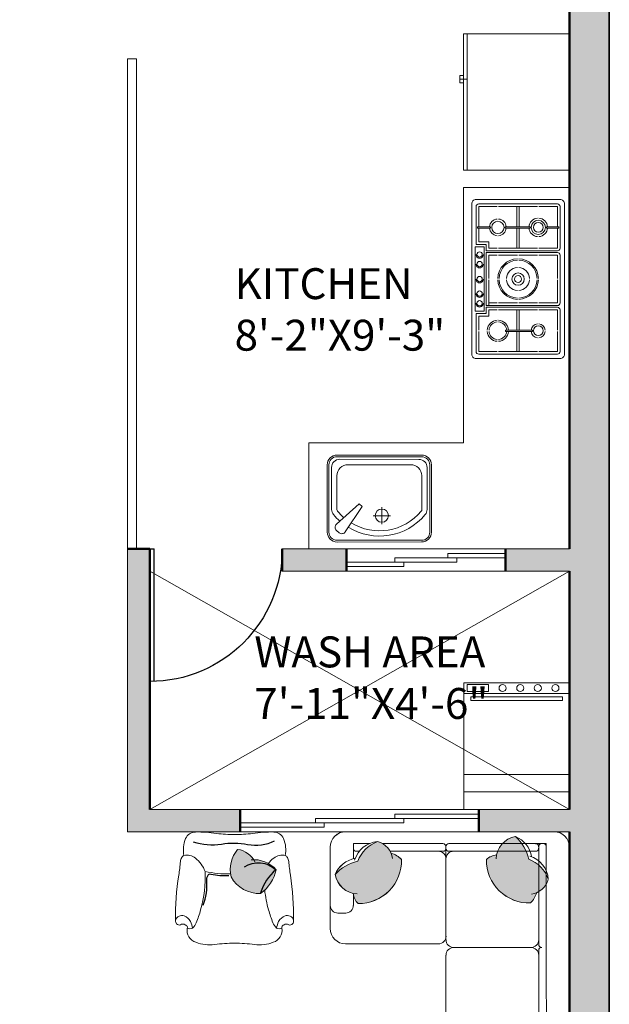
# Model space of a CAD drawing. Units: inches. Extents: x 1734 to 4011, y 1071 to 1891.
# Tile 17 of 27: x 3343 to 3476, y 1415 to 1638. Entities that reach past the tile are written whole.
import ezdxf

# ---------------------------------------------------------------- set-up
doc = ezdxf.new("R2010")
doc.units = ezdxf.units.IN
for name, color, linetype, lineweight in [('A-AREA-IDEN', 3, 'Continuous', 18), ('A-DOOR', 3, 'Continuous', 25), ('A-EQPM', 8, 'Continuous', 18), ('A-FLOR-FIXT', 9, 'Continuous', 18), ('A-FURN', 8, 'Continuous', 18), ('A-FURN-PATT', 252, 'Continuous', 13), ('A-GLAZ', 4, 'Continuous', 18), ('A-WALL', 7, 'Continuous', 50), ('A-WALL-PATT', 8, 'Continuous', 13), ('C-PROP', 1, 'Continuous', 35)]:
    doc.layers.add(name, color=color, linetype=linetype, lineweight=lineweight)
doc.layers.add('IFF-FURN-DETAIL', color=250, linetype='Continuous')
doc.styles.get("Standard").update_dxf_attribs({"font": 'arial.ttf'})

# ---------------------------------------------------------------- blocks, each defined once
blk = doc.blocks.new('STOVE')
for p, q in [((11.85, 19.7), (11.55, 19.7)), ((11.55, 16.92), (11.55, 19.7)), ((11.85, 16.92), (11.85, 19.7)), ((11.85, 16.92), (11.55, 16.92)), ((-11.85, 13.73), (-11.85, 7.62)), ((-11.85, 13.73), (-11.55, 13.73)), ((-11.55, 13.73), (-11.55, 7.62)), ((11.85, 13.23), (11.55, 13.23)), ((11.55, 13.23), (11.55, 7.57)), ((11.85, 13.23), (11.85, 7.57)), ((-11.85, 10.75), (-16.4, 10.75)), ((-11.85, 10.25), (-16.4, 10.25)), ((-7, 10.75), (-11.55, 10.75)), ((-7, 10.25), (-11.55, 10.25)), ((7, 10.75), (11.55, 10.75)), ((7, 10.25), (11.55, 10.25)), ((11.85, 10.75), (16.4, 10.75)), ((11.85, 10.25), (16.4, 10.25)), ((-11.85, 7.62), (-11.55, 7.62)), ((11.85, 7.57), (11.55, 7.57)), ((-7, 3.9), (-8.4, 3.9)), ((-7.8, 3.3), (-7.8, 1)), ((-6.4, 3.3), (-7.8, 3.3)), ((7.3, 2.8), (-7.3, 2.8)), ((-7.3, 2.8), (-7.3, 0.8)), ((-5.4, 3.9), (-6, 3.9)), ((-5.4, 3.9), (-0.15, 3.9)), ((0.15, 3.9), (5.4, 3.9)), ((6.4, 3.3), (7.8, 3.3)), ((7, 3.9), (8.4, 3.9)), ((7.3, 2.8), (7.3, 0.8)), ((7.8, 3.3), (7.8, 1)), ((8.4, 3.9), (8.4, 1.6)), ((11.85, 4.28), (11.55, 4.28)), ((11.55, 4.28), (11.55, 1.3)), ((11.85, 4.28), (11.85, 1.3)), ((7.3, 0.8), (-7.3, 0.8)), ((11.85, 1.3), (11.55, 1.3))]:
    blk.add_line(p, q)
for points in [[(-17, 21), (17, 21, -0.414214), (18, 20), (18, 1, -0.414214), (17, 0), (-17, 0, -0.414214), (-18, 1), (-18, 20, -0.414214)], [(6, 3.3), (-6, 3.3), (-6, 19.4, -0.414214), (-5.4, 20), (5.4, 20, -0.414214), (6, 19.4)]]:
    blk.add_lwpolyline(points, format="xyb", close=True)
for points in [[(-7.8, 1), (-16.4, 1, -0.414214), (-17, 1.6), (-17, 19.4, -0.414214), (-16.4, 20), (-7, 20, -0.414214), (-6.4, 19.4), (-6.4, 3.3)], [(6.4, 19.4, -0.414214), (7, 20), (16.4, 20, -0.414214), (17, 19.4), (17, 1.6, -0.414214), (16.4, 1), (7.8, 1)]]:
    blk.add_lwpolyline(points, format="xyb")
for points in [[(-16.4, 15.22), (-16.4, 19.4), (-11.85, 19.4)], [(-11.55, 19.4), (-7, 19.4), (-7, 15.22)], [(-5.4, 15.22), (-5.4, 19.4), (-0.15, 19.4)], [(0.15, 19.4), (5.4, 19.4), (5.4, 15.22)], [(6.4, 3.3), (6.4, 19.4)], [(7, 15.22), (7, 19.4), (11.55, 19.4)], [(11.85, 19.4), (16.4, 19.4), (16.4, 15.22)], [(-16.4, 6.08), (-16.4, 14.92)], [(-7, 14.92), (-7, 6.08)], [(-5.4, 10.65), (-5.4, 14.92)], [(5.4, 14.92), (5.4, 10.65)], [(7, 6.08), (7, 14.92)], [(16.4, 14.92), (16.4, 6.08)], [(-5.4, 6.08), (-5.4, 10.35)], [(5.4, 10.35), (5.4, 6.08)], [(-11.85, 1.6), (-16.4, 1.6), (-16.4, 5.77)], [(-7, 5.77), (-7, 3.9)], [(-5.4, 3.9), (-5.4, 5.77)], [(5.4, 5.77), (5.4, 3.9)], [(7, 3.9), (7, 5.77)], [(16.4, 5.77), (16.4, 1.6), (11.85, 1.6)], [(-8.4, 3.9), (-8.4, 1.6), (-11.55, 1.6)], [(11.55, 1.6), (8.4, 1.6)]]:
    blk.add_lwpolyline(points)
for centre, radius in [((-11.7, 15.07), 1.1), ((11.7, 15.07), 1.6), ((11.7, 15.07), 1.1), ((0, 10.5), 1.4), ((0, 10.5), 0.8), ((11.7, 5.93), 1.4), ((-5.49, 1.8), 0.6), ((-3.3, 1.8), 0.6), ((0, 1.8), 0.6), ((3.39, 1.8), 0.6), ((5.57, 1.8), 0.6)]:
    blk.add_circle(centre, radius)
for centre, radius, start, end in [((-11.7, 15.07), 1.6, 95.3794, 174.6206), ((-11.7, 15.07), 1.6, 5.3794, 84.6206), ((11.7, 15.07), 2.1, 94.096, 175.904), ((11.7, 15.07), 2.1, 4.096, 85.904), ((-11.7, 15.07), 1.6, 185.3794, 264.6206), ((-11.7, 15.07), 1.6, 275.3794, 354.6206), ((0, 10.5), 4.6, 91.8687, 178.1313), ((0, 10.5), 4.3, 91.9991, 178.0009), ((0, 10.5), 4.6, 1.8687, 88.1313), ((0, 10.5), 4.3, 1.9991, 88.0009), ((11.7, 15.07), 2.1, 184.096, 265.904), ((11.7, 15.07), 2.1, 274.096, 355.904), ((0, 10.5), 2.6, 93.3074, 176.6926), ((0, 10.5), 2.6, 3.3074, 86.6926), ((0, 10.5), 4.6, 181.8687, 268.1313), ((0, 10.5), 4.3, 181.9991, 268.0009), ((0, 10.5), 2.6, 183.3074, 266.6926), ((0, 10.5), 4.6, 271.8687, 358.1313), ((0, 10.5), 4.3, 271.9991, 358.0009), ((0, 10.5), 2.6, 273.3074, 356.6926), ((-11.7, 5.93), 2.4, 93.5833, 176.4167), ((-11.7, 5.93), 2, 94.3012, 175.6988), ((-11.7, 5.93), 2.4, 3.5833, 86.4167), ((-11.7, 5.93), 2, 4.3012, 85.6988), ((11.7, 5.93), 1.9, 94.5281, 175.4719), ((11.7, 5.93), 1.9, 4.5281, 85.4719), ((-11.7, 5.93), 2.4, 183.5833, 266.4167), ((-11.7, 5.93), 2, 184.3012, 265.6988), ((-11.7, 5.93), 2.4, 273.5833, 356.4167), ((-11.7, 5.93), 2, 274.3012, 355.6988), ((11.7, 5.93), 1.9, 184.5281, 265.4719), ((11.7, 5.93), 1.9, 274.5281, 355.4719), ((-5.49, 1.8), 0.846, 89.9979, 270), ((-3.3, 1.8), 0.846, 89.9979, 270), ((0, 1.8), 0.846, 89.9979, 270), ((3.39, 1.8), 0.846, 89.9979, 270), ((5.57, 1.8), 0.846, 89.9979, 270)]:
    blk.add_arc(centre, radius, start, end)
blk = doc.blocks.new('Refrigerator-2 door - 36 in top')
for p, q in [((0, -26.999999), (36, -26.999999)), ((11, -27.999999), (11, -28.999999)), ((12, -26.999999), (12, -28.999999)), ((13, -28.999999), (13, -27.999999)), ((11, -28.999999), (13, -28.999999))]:
    blk.add_line(p, q)
blk.add_lwpolyline([(0, -27.999999), (0, 0), (36, 0), (36, -27.999999)], close=True)
blk = doc.blocks.new("D2 2'6")
for p, q in [((0, 30), (0, 0)), ((1, 30), (1, 0)), ((0, 0), (1, 0))]:
    blk.add_line(p, q)
blk.add_arc((0, 0), 30, 0, 90)
blk = doc.blocks.new('SOFA 1')
at = {"transparency": 33554687}
h = blk.add_hatch(color=256, dxfattribs=at)
h.dxf.hatch_style = 1
h.paths.add_polyline_path([(3723.52, 1308.63, 0.147724), (3717.76, 1305.24, 0.310469), (3722.42, 1300.4), (3722.42, 1300.25, 0.156703), (3723.62, 1297.8, 0.425821), (3734.69, 1309.08, 0.121928), (3732.05, 1310.63, 0.233216), (3728.6, 1313.59, 0.213835)])
h = blk.add_hatch(color=256, dxfattribs=at)
h.dxf.hatch_style = 1
h.paths.add_polyline_path([(3769.65, 1307.6, 0.084911), (3767.15, 1309.12, 0.046133), (3766.46, 1311.13), (3759.18, 1311.13, 0.039409), (3758.92, 1310.24, 0.165523), (3756.31, 1309.02, 0.42585), (3767.59, 1297.95, 0.121928), (3769.15, 1300.58, 0.027403), (3769.65, 1300.83)])
h.paths.add_polyline_path([(3765.34, 1313.08), (3760.4, 1313.08, 0.097704), (3759.18, 1311.13), (3766.46, 1311.13, 0.04873)])
h.paths.add_polyline_path([(3763.76, 1314.88, 0.16488), (3760.4, 1313.08), (3765.34, 1313.08, 0.051917)])
h.paths.add_polyline_path([(3771.6, 1305.17, 0.090388), (3769.65, 1307.6), (3769.65, 1300.83, 0.136035), (3771.6, 1302.77)])
h = blk.add_hatch(color=256, dxfattribs=at)
h.dxf.hatch_style = 1
h.paths.add_polyline_path([(3769.16, 1235.96, 0.122267), (3767.6, 1238.61, 0.425972), (3756.32, 1227.54, 0.165563), (3758.93, 1226.32, 0.309481), (3763.76, 1221.69, 0.002677), (3763.83, 1221.72, 0.146094), (3767.16, 1227.43, 0.212433), (3772.1, 1232.48, 0.235342)])
h = blk.add_hatch(color=256, dxfattribs=at)
h.dxf.hatch_style = 1
h.paths.add_polyline_path([(3769.16, 1225.36, 0.122267), (3767.6, 1228.01, 0.425972), (3756.32, 1216.94, 0.165563), (3758.93, 1215.72, 0.309481), (3763.76, 1211.09, 0.002677), (3763.83, 1211.12, 0.146094), (3767.16, 1216.83, 0.212433), (3772.1, 1221.88, 0.235342)])
for p, q in [((3720.45, 1316.13), (3773.58, 1316.13)), ((3777.51, 1312.19), (3777.51, 1213.72))]:
    blk.add_line(p, q, dxfattribs=at)
for points in [[(3717.76, 1305.24, -0.147724), (3723.52, 1308.63, -0.213355), (3728.59, 1313.59, 0.213355), (3723.52, 1308.63, 0.147724), (3717.76, 1305.24, -0.249545), (3722.86, 1309.34, 0.249545), (3717.75, 1305.25, 0.356779), (3723.4, 1300.28, -0.356779), (3717.76, 1305.24)], [(3728.58, 1313.6, -0.306333), (3732.42, 1309.31, 0.306333), (3728.58, 1313.6, 0.306674), (3722.72, 1308.89, -0.306674), (3728.58, 1313.6)], [(3763.76, 1314.88, -0.147724), (3767.15, 1309.12, -0.213355), (3772.1, 1304.05, 0.213355), (3767.15, 1309.12, 0.147724), (3763.76, 1314.88, -0.249545), (3767.86, 1309.77, 0.249545), (3763.77, 1314.89, 0.356779), (3758.8, 1309.23, -0.356779), (3763.76, 1314.88)], [(3734.69, 1309.08, -0.425972), (3723.62, 1297.8, -0.165552), (3722.4, 1300.4, 0.165552), (3723.62, 1297.79, 0.425972), (3734.69, 1309.07, 0.121514), (3732.07, 1310.63, -0.121514), (3734.69, 1309.08)], [(3767.6, 1297.95, -0.425972), (3756.31, 1309.01, -0.165552), (3758.92, 1310.24, 0.165552), (3756.31, 1309.02, 0.425972), (3767.59, 1297.95, 0.121514), (3769.14, 1300.57, -0.121514), (3767.6, 1297.95)], [(3772.11, 1304.06, -0.306333), (3767.83, 1300.22, 0.306333), (3772.11, 1304.06, 0.306674), (3767.4, 1309.91, -0.306674), (3772.11, 1304.06)], [(3770.44, 1286.63, -0.414214), (3769.66, 1287.4, 0.414214), (3770.44, 1286.63, 0.414214), (3769.66, 1285.83, -0.414214), (3770.44, 1286.63)], [(3748.01, 1262.99, -0.414214), (3746.05, 1264.95, 0.414214), (3748.01, 1262.97, 0.414213), (3746.05, 1261.01, -0.414213), (3748.01, 1262.99)], [(3770.44, 1262.99, -0.414214), (3769.66, 1263.77, 0.414214), (3770.44, 1262.99, 0.414214), (3769.66, 1262.19, -0.414214), (3770.44, 1262.99)], [(3770.83, 1262.97, -0.414214), (3771.61, 1262.19, 0.414214), (3770.83, 1262.99, 0.414214), (3771.61, 1263.77, -0.414214), (3770.83, 1262.97)], [(3748.01, 1239.35, -0.414214), (3746.05, 1241.31, 0.414214), (3748.01, 1239.33, 0.414213), (3746.05, 1237.37, -0.414213), (3748.01, 1239.35)], [(3767.7, 1239.33, -0.414214), (3769.66, 1237.37, 0.414214), (3767.7, 1239.35, 0.414214), (3769.66, 1241.31, -0.414214), (3767.7, 1239.33)], [(3756.32, 1227.54, -0.425972), (3767.6, 1238.61, -0.121514), (3769.16, 1235.98, 0.121514), (3767.6, 1238.61, 0.425972), (3756.32, 1227.54, 0.165552), (3758.93, 1226.32, -0.165552), (3756.32, 1227.54)], [(3770.44, 1239.35, -0.414214), (3769.66, 1240.13, 0.414214), (3770.44, 1239.33, 0.414214), (3769.66, 1238.55, -0.414214), (3770.44, 1239.35)], [(3770.83, 1239.33, -0.414214), (3771.61, 1238.55, 0.414214), (3770.83, 1239.35, 0.414214), (3771.61, 1240.13, -0.414214), (3770.83, 1239.33)], [(3772.1, 1232.5, -0.306674), (3767.41, 1226.64, 0.306674), (3772.1, 1232.5, 0.306333), (3767.84, 1236.34, -0.306333), (3772.1, 1232.5)], [(3763.78, 1221.67, 0.249545), (3767.87, 1226.78, -0.249545), (3763.76, 1221.69, -0.356779), (3758.81, 1227.32, 0.356779), (3763.77, 1221.68, 0.147724), (3767.16, 1227.43, 0.213355), (3772.11, 1232.51, -0.213355), (3767.16, 1227.43, -0.147724), (3763.78, 1221.67)], [(3756.32, 1216.94, -0.200233), (3759.49, 1224.76, 0.200233), (3756.32, 1216.94, 0.165552), (3758.93, 1215.72, -0.165552), (3756.32, 1216.94)], [(3772.1, 1221.9, -0.306674), (3767.41, 1216.04, 0.306674), (3772.1, 1221.9, -0.213355), (3767.16, 1216.83, -0.147724), (3763.77, 1211.08, 0.147724), (3767.15, 1216.83, 0.213355), (3772.1, 1221.9)], [(3763.76, 1211.09, -0.356779), (3758.81, 1216.72, 0.356779), (3763.76, 1211.09, 0.249545), (3767.87, 1216.18, -0.249545), (3763.76, 1211.09)]]:
    blk.add_lwpolyline(points, format="xyb", dxfattribs=at)
for points in [[(3716.51, 1312.2), (3716.51, 1291.44)], [(3722.42, 1313.08), (3722.42, 1309.23), (3722.42, 1313.08), (3726.57, 1313.08)], [(3723.21, 1311.13), (3723.93, 1311.13)], [(3729.85, 1313.08), (3745.25, 1313.08)], [(3731.82, 1311.13), (3745.25, 1311.13)], [(3746.01, 1312.3), (3746.01, 1288.55)], [(3746.01, 1310.97), (3746.01, 1311.36)], [(3768.11, 1313.08), (3746.78, 1313.08)], [(3768.87, 1311.13), (3746.78, 1311.13)], [(3771.6, 1313.08), (3767.75, 1313.08), (3771.6, 1313.08), (3771.6, 1308.93)], [(3769.66, 1287.39), (3769.65, 1312.3)], [(3771.6, 1313.08), (3771.61, 1233.74)], [(3769.65, 1309.43), (3769.65, 1308.71)], [(3746.01, 1288.54), (3746.01, 1308.23)], [(3722.42, 1300.39), (3722.42, 1297.33)], [(3720.45, 1295.38), (3718.48, 1295.38)], [(3720.45, 1287.5), (3744.09, 1287.5)], [(3747.99, 1286.6), (3767.69, 1286.6)], [(3769.66, 1263.75), (3769.66, 1285.81)], [(3746.02, 1284.63), (3746.02, 1264.94)], [(3769.66, 1277.18), (3769.66, 1263.75)], [(3746.02, 1260.99), (3746.02, 1241.3)], [(3747.99, 1262.97), (3767.69, 1262.97)], [(3769.66, 1240.12), (3769.66, 1262.18)], [(3770.43, 1262.97), (3770.82, 1262.97)], [(3747.99, 1239.33), (3767.69, 1239.33)], [(3769.66, 1235.71), (3769.66, 1238.54)], [(3770.43, 1239.33), (3770.82, 1239.33)], [(3746.02, 1237.36), (3746.02, 1213.74)], [(3771.61, 1223.14), (3771.61, 1230.47)], [(3769.66, 1225.11), (3769.66, 1227.82)], [(3767.76, 1215.72), (3771.61, 1215.72), (3771.61, 1219.84), (3771.61, 1215.72)], [(3755.86, 1215.72), (3758.92, 1215.72)], [(3769.66, 1216.5), (3769.66, 1217.22)], [(3753.91, 1211.77), (3753.91, 1213.74)], [(3749.97, 1209.8), (3773.58, 1209.8)]]:
    blk.add_lwpolyline(points, close=True, dxfattribs=at)
for points in [[(3722.42, 1311.91, 0.414214), (3723.2, 1311.13, -0.414214)], [(3770.43, 1313.08, 0.414214), (3769.65, 1312.3, -0.414214)], [(3771.6, 1312.3, 0.414214), (3770.82, 1313.08, -0.414214)], [(3716.51, 1297.34, 0.414214), (3718.47, 1295.38, -0.414214)], [(3720.44, 1295.38, 0.414214), (3722.4, 1297.34, -0.414214)], [(3716.51, 1291.45, 0.414212), (3720.44, 1287.52, -0.414212)], [(3746.03, 1288.56, 0.414214), (3747.99, 1286.6, 0.414213), (3746.03, 1284.64, -0.414213), (3747.99, 1286.6, -0.414214)], [(3769.66, 1284.64, 0.414214), (3767.7, 1286.6, 0.414214), (3769.66, 1288.56, -0.414214), (3767.7, 1286.6, -0.414214)], [(3769.66, 1261.01, 0.414214), (3767.7, 1262.97, 0.414214), (3769.66, 1264.93, -0.414214), (3767.7, 1262.97, -0.414214)], [(3772.13, 1221.9, 0.306333), (3767.84, 1225.74, -0.306333)], [(3769.16, 1225.36, 0.071861), (3768.39, 1227.01, -0.071861)], [(3755.87, 1215.72, 0.414214), (3753.91, 1213.76, -0.414214)], [(3769.66, 1216.52, 0.414214), (3770.44, 1215.74, -0.414214)], [(3770.83, 1215.74, 0.414214), (3771.61, 1216.52, -0.414214)], [(3746.05, 1213.76, 0.414212), (3749.98, 1209.82, -0.414212)], [(3755.87, 1209.8, -0.414214), (3753.91, 1211.76, 0.414214)]]:
    blk.add_lwpolyline(points, format="xyb", close=True, dxfattribs=at)
for centre, radius, start, end in [((3720.44, 1312.2), 3.93, 90.0002, 179.9998), ((3720.44, 1312.19), 3.94, 89.9158, 179.9154), ((3773.58, 1312.2), 3.93, 0.0002, 89.9998), ((3773.57, 1312.19), 3.94, 359.9158, 89.9154), ((3744.09, 1309.21), 1.92, 358.766, 90.5111), ((3745.22, 1312.29), 0.789, 0.8425, 90.8425), ((3745.24, 1311.91), 0.777, 270, 0), ((3745.24, 1311.91), 0.777, 270, 0), ((3746.8, 1312.29), 0.789, 89.1575, 179.1575), ((3746.79, 1311.91), 0.777, 180, 270), ((3746.79, 1311.91), 0.777, 180, 270), ((3747.93, 1309.21), 1.92, 89.4889, 181.234), ((3768.87, 1312.3), 0.777, 360, 90), ((3768.87, 1311.91), 0.777, 270, 0), ((3744.08, 1289.48), 1.96, 270, 360), ((3744.08, 1289.48), 1.96, 270, 360), ((3773.58, 1213.73), 3.93, 270.0002, 359.9998), ((3773.59, 1213.73), 3.93, 269.9156, 359.9152)]:
    blk.add_arc(centre, radius, start, end, dxfattribs=at)
blk = doc.blocks.new('PILLOW-1')
at = {"color": 0}
blk.add_lwpolyline([(198, -165.3, -0.232884), (126.3, -346, -0.184752), (-44.3, -233.7, -0.286563), (74.8, -22, -0.237978), (272.6, -68.2, -0.243587), (179.4, -195.4, 4.263709)], format="xyb", dxfattribs=at)
at = {"layer": 'IFF-FURN-DETAIL'}
blk.add_lwpolyline([(147.6, -117.6, -0.343333), (126.5, -342.2, 0.126408), (-39.5, -232.6, -5.969376)], format="xyb", dxfattribs=at)
blk = doc.blocks.new('CLNG90')
for points in [[(689.4, 369.7, 0.157831), (676.6, 385.2, 0.121013), (646.4, 395.4, -0.017334), (546.8, 407.4, 0.041496), (215.3, 431.2, 0.153531), (191.4, 423.4, 0.382906), (185.1, 395.3, -0.284047), (183.7, 360.8, 0.011997), (177.2, 350.7, -0.370479), (159.9, 345, 0.380647), (56.2, 282, 0.117468), (40.6, 145.8, -0.027775), (50, 0, -8.773898)], [(159.9, 345, 0.22481), (159.8, 306.3, 0.055398), (209.2, 321.6, 0.180116), (248.9, 368.2, 0.194833), (247.6, 405.4, 0.242377), (215.3, 431.2, 1.52074)], [(159.9, 345, 0.22481), (159.8, 306.3, 0.055398), (209.2, 321.6, 0.180116), (248.9, 368.2, 0.194833), (247.6, 405.4, 0.242377), (215.3, 431.2, 1.52074)], [(689.4, 369.7, -0.235486), (671.3, 286, -0.134038), (573.9, 215.1, -0.079303), (292.9, 247.8, -0.027048), (199.2, 279.7, -0.106276), (159.8, 306.3, -1.699)], [(689.4, 369.7, -0.235486), (671.3, 286, -0.134038), (573.9, 215.1, -0.079303), (292.9, 247.8, -0.027048), (199.2, 279.7, -0.106276), (159.8, 306.3, -1.699)], [(689.4, 369.7, -0.146607), (813.9, 357.3, -0.305296), (861.7, 285.6, -0.042137), (851.9, 131.4, 0.040285), (843.1, 0, 3.952121)], [(573.9, 215.1, 0.061244), (555.6, 29, 3.376255)], [(573.9, 215.1, 0.061244), (555.6, 29, 3.376255)], [(689.4, -369.7, -0.157831), (676.6, -385.2, -0.121013), (646.4, -395.4, 0.017334), (546.8, -407.4, -0.041496), (215.3, -431.2, -0.153531), (191.4, -423.4, -0.382906), (185.1, -395.3, 0.284047), (183.7, -360.8, -0.011997), (177.2, -350.7, 0.370479), (159.9, -345, -0.380647), (56.2, -282, -0.117468), (40.6, -145.8, 0.027775), (50, 0, 8.773898)], [(689.4, -369.7, 0.146607), (813.9, -357.3, 0.305296), (861.7, -285.6, 0.042137), (851.9, -131.4, -0.040285), (843.1, 0, -3.952121)], [(437.4, -219.7, 0.041086), (292.9, -247.8, 0.027048), (199.2, -279.7, 0.106276), (159.8, -306.3, 1.699)], [(437.4, -219.7, 0.041086), (292.9, -247.8, 0.027048), (199.2, -279.7, 0.106276), (159.8, -306.3, 1.699)], [(689.4, -369.7, 0.235486), (671.3, -286, 0.060693), (631.8, -247.3, 0.001296)], [(689.4, -369.7, 0.235486), (671.3, -286, 0.060693), (631.8, -247.3, 0.001296)], [(159.9, -345, -0.22481), (159.8, -306.3, -0.055398), (209.2, -321.6, -0.180116), (248.9, -368.2, -0.194833), (247.6, -405.4, -0.242377), (215.3, -431.2, -1.52074)], [(159.9, -345, -0.22481), (159.8, -306.3, -0.055398), (209.2, -321.6, -0.180116), (248.9, -368.2, -0.194833), (247.6, -405.4, -0.242377), (215.3, -431.2, -1.52074)]]:
    blk.add_lwpolyline(points, format="xyb")
at = {"layer": 'IFF-FURN-DETAIL'}
for points in [[(790.6, 301.1, 0.124986), (773.9, 95.7, -0.091334), (771.1, -94.9, 0.164688), (796.9, -292.4, 1.068868)], [(790.6, 301.1, 0.124986), (773.9, 95.7, -0.091334), (771.1, -94.9, 0.164688), (796.9, -292.4, 1.068868)], [(328.2, 228.3, 0.109125), (508.5, 203.4, -0.16587), (546, 193.9, -0.314359), (554.8, 172.3, 0.072017), (544.2, 42.1, 4.351186)], [(328.2, 228.3, 0.109125), (508.5, 203.4, -0.16587), (546, 193.9, -0.314359), (554.8, 172.3, 0.072017), (544.2, 42.1, 4.351186)]]:
    blk.add_lwpolyline(points, format="xyb", dxfattribs=at)
at = {"xscale": 1.016, "yscale": 1.016, "zscale": 1.016}
blk.add_blockref('PILLOW-1', (458.1, 47.3), dxfattribs=at)
blk.add_blockref('PILLOW-1', (458.1, 47.3), dxfattribs=at)
blk = doc.blocks.new('Range-Oven - 30 in front')
for p, q in [((0, 33.00005), (30, 33.00005)), ((30, 10), (0, 10)), ((0, 5), (30, 5))]:
    blk.add_line(p, q)
for points in [[(0, 0), (0, 36.00005), (30, 36.00005), (30, 0)], [(1, 33.50005), (1, 35.50005), (7, 35.50005), (7, 33.50005)], [(2, 31.00005), (2, 32.00005), (28, 32.00005), (28, 31.00005)]]:
    blk.add_lwpolyline(points, close=True)
for centre in [(11, 34.50005), (16, 34.50005), (21, 34.50005), (26, 34.50005)]:
    blk.add_circle(centre, 1)

msp = doc.modelspace()

# ---------------------------------------------------------------- hatches: boundary and pattern name
at = {"layer": 'A-FURN-PATT'}
h = msp.add_hatch(color=256, dxfattribs=at)
h.dxf.hatch_style = 1
h.paths.add_polyline_path([(3397.1, 1439.84, 0.184752), (3400.63, 1445.21, 0.210353), (3395.54, 1447.49, 0.209279), (3391.88, 1449.82, 0.237978), (3390.43, 1443.59, 0.286563)])
at = {"layer": 'A-WALL-PATT'}
h = msp.add_hatch(color=256, dxfattribs=at)
h.dxf.hatch_style = 1
h.paths.add_polyline_path([(3475.99, 1831.82), (3115.99, 1831.82), (3115.99, 1745.82), (3130.99, 1745.82), (3130.99, 1750.82), (3124.99, 1750.82), (3124.99, 1822.82), (3214.99, 1822.82), (3214.99, 1780.82), (3219.99, 1780.82), (3219.99, 1822.82), (3308.99, 1822.82), (3308.99, 1750.82), (3254.99, 1750.82), (3254.99, 1745.82), (3308.99, 1745.82), (3308.99, 1604.82), (3313.99, 1604.82), (3313.99, 1745.82), (3366.99, 1745.82), (3366.99, 1750.82), (3313.99, 1750.82), (3313.99, 1822.82), (3401.99, 1822.82), (3401.99, 1750.82), (3396.99, 1750.82), (3396.99, 1745.82), (3411.99, 1745.82), (3411.99, 1750.82), (3406.99, 1750.82), (3406.99, 1822.82), (3466.99, 1822.82), (3466.99, 1750.82), (3441.99, 1750.82), (3441.99, 1745.82), (3466.99, 1745.82), (3466.99, 1517.82), (3452.49, 1517.82), (3452.49, 1512.82), (3466.99, 1512.82), (3466.99, 1458.82), (3446.49, 1458.82), (3446.49, 1453.82), (3466.99, 1453.82), (3466.99, 1237.82), (3372.99, 1237.82), (3372.99, 1228.82), (3466.99, 1228.82), (3466.99, 1120.82), (3309.99, 1120.82), (3309.99, 1184.82), (3310.99, 1184.82), (3310.99, 1189.82), (3303.99, 1189.82), (3303.99, 1120.82), (3291.99, 1120.82), (3291.99, 1111.82), (3475.99, 1111.82)])
h.paths.add_polyline_path([(3169.99, 1745.82), (3224.99, 1745.82), (3224.99, 1750.82), (3154.99, 1750.82), (3154.99, 1745.82), (3160.99, 1745.82), (3160.99, 1636.82), (3169.99, 1636.82)], flags=17)
h.paths.add_polyline_path([(3169.99, 1588.82), (3160.99, 1588.82), (3160.99, 1559.82), (3313.99, 1559.82), (3313.99, 1568.82), (3308.99, 1568.82), (3308.99, 1564.82), (3169.99, 1564.82)], flags=17)
h.paths.add_polyline_path([(3416.49, 1517.82), (3401.99, 1517.82), (3401.99, 1512.82), (3416.49, 1512.82)], flags=17)
h.paths.add_polyline_path([(3371.99, 1517.82), (3366.99, 1517.82), (3366.99, 1453.82), (3392.49, 1453.82), (3392.49, 1458.82), (3371.99, 1458.82)], flags=17)
h.paths.add_polyline_path([(3258.99, 1529.82), (3160.99, 1529.82), (3160.99, 1494.82), (3169.99, 1494.82), (3169.99, 1524.82), (3253.99, 1524.82), (3253.99, 1520.82), (3258.99, 1520.82)], flags=17)
h.paths.add_polyline_path([(3263.99, 1458.82), (3258.99, 1458.82), (3258.99, 1490.82), (3253.99, 1490.82), (3253.99, 1458.82), (3169.99, 1458.82), (3169.99, 1470.82), (3160.99, 1470.82), (3160.99, 1387.82), (3169.99, 1387.82), (3169.99, 1453.82), (3263.99, 1453.82)], flags=17)
h.paths.add_polyline_path([(3313.99, 1453.82), (3318.99, 1453.82), (3318.99, 1458.82), (3299.99, 1458.82), (3299.99, 1453.82), (3308.99, 1453.82), (3308.99, 1321.82), (3266.49, 1321.82), (3266.49, 1312.82), (3313.99, 1312.82)], flags=17)
h.paths.add_polyline_path([(3212.49, 1321.82), (3169.99, 1321.82), (3169.99, 1339.82), (3160.99, 1339.82), (3160.99, 1312.82), (3212.49, 1312.82)], flags=17)
h.paths.add_polyline_path([(3313.99, 1288.82), (3304.99, 1288.82), (3304.99, 1285.82), (3313.99, 1285.82)], flags=17)
h.paths.add_polyline_path([(3324.99, 1237.82), (3304.99, 1237.82), (3304.99, 1228.82), (3324.99, 1228.82)], flags=17)

# ---------------------------------------------------------------- linework, layer by layer
at = {"layer": 'A-FLOR-FIXT'}
msp.add_circle((3424.51, 1525.37), 1.5, dxfattribs=at)
at = {"layer": 'A-FURN'}
for p, q in [((3366.99, 1628.82), (3368.99, 1628.82)), ((3366.99, 1628.82), (3366.99, 1453.82)), ((3368.99, 1628.82), (3368.99, 1517.82)), ((3442.99, 1599.69), (3442.99, 1541.82)), ((3442.99, 1599.69), (3466.99, 1599.69)), ((3407.99, 1541.82), (3442.99, 1541.82)), ((3407.99, 1541.82), (3407.99, 1517.82)), ((3401.99, 1517.82), (3466.99, 1517.82)), ((3466.99, 1512.82), (3371.99, 1458.82)), ((3371.99, 1512.82), (3466.99, 1458.82)), ((3401.99, 1512.82), (3466.99, 1512.82)), ((3371.99, 1458.82), (3466.99, 1458.82)), ((3366.99, 1453.82), (3466.99, 1453.82))]:
    msp.add_line(p, q, dxfattribs=at)
for points in [[(3414.4, 1539.09, 0.414214), (3412.16, 1536.86), (3412.18, 1521.64, 0.414214), (3414.39, 1519.4), (3433.53, 1519.42, 0.414214), (3435.75, 1521.62), (3435.75, 1536.86, 0.414214), (3433.52, 1539.09), (3414.4, 1539.09)], [(3414.4, 1538.72, 0.414214), (3412.55, 1536.86), (3412.55, 1521.64, 0.414214), (3414.39, 1519.79), (3433.53, 1519.79, 0.414214), (3435.36, 1521.62), (3435.36, 1536.86, 0.414214), (3433.52, 1538.7), (3414.4, 1538.72)], [(3416.92, 1522.74, 0.371519), (3434.35, 1525.6, 0.175764), (3434.75, 1526.77), (3434.78, 1536.27, 0.414214), (3432.92, 1538.09), (3415, 1538.12, 0.414214), (3413.16, 1536.26), (3413.16, 1526.77, 0.175764), (3413.59, 1525.6, 0.038632), (3415.04, 1524.12)], [(3417.57, 1523.73, 0.370401), (3433.44, 1526.36, 0.175764), (3433.57, 1526.77), (3433.57, 1534.42, 0.414214), (3431.06, 1536.91), (3416.86, 1536.91, 0.414214), (3414.34, 1534.41), (3414.34, 1526.77, 0.175764), (3414.49, 1526.36, 0.038512), (3415.93, 1524.91)]]:
    msp.add_lwpolyline(points, format="xyb", dxfattribs=at)
msp.add_lwpolyline([(3414.27, 1522), (3414.85, 1521.51, 0.463205), (3416.24, 1521.72), (3420.07, 1527.45), (3419.37, 1528.05), (3414.29, 1523.41, 0.4637)], format="xyb", close=True, dxfattribs=at)
for points in [[(3424.5, 1523.41), (3424.5, 1527.31)], [(3426.45, 1525.36), (3422.55, 1525.36)]]:
    msp.add_lwpolyline(points, dxfattribs=at)
at = {"layer": 'A-GLAZ'}
for p, q in [((3427.49, 1514.82), (3427.49, 1515.82)), ((3427.49, 1515.82), (3452.49, 1515.82)), ((3439.49, 1515.82), (3439.49, 1516.82)), ((3439.49, 1516.82), (3452.49, 1516.82)), ((3441.49, 1514.82), (3441.49, 1515.82)), ((3416.49, 1514.82), (3441.49, 1514.82)), ((3416.49, 1513.82), (3429.49, 1513.82)), ((3429.49, 1513.82), (3429.49, 1514.82)), ((3427.49, 1457.82), (3427.49, 1456.82)), ((3427.49, 1457.82), (3446.49, 1457.82)), ((3392.49, 1455.82), (3429.49, 1455.82)), ((3409.49, 1456.82), (3409.49, 1455.82)), ((3409.49, 1456.82), (3446.49, 1456.82)), ((3411.49, 1455.82), (3411.49, 1454.82)), ((3429.49, 1456.82), (3429.49, 1455.82)), ((3392.49, 1454.82), (3411.49, 1454.82))]:
    msp.add_line(p, q, dxfattribs=at)
at = {"layer": 'A-WALL'}
for p, q in [((3466.99, 1745.82), (3466.99, 1517.82)), ((3366.99, 1517.82), (3371.99, 1517.82)), ((3371.99, 1517.82), (3371.99, 1458.82)), ((3401.99, 1517.82), (3401.99, 1512.82)), ((3416.49, 1512.82), (3416.49, 1517.82)), ((3452.49, 1512.82), (3452.49, 1517.82)), ((3466.99, 1512.82), (3466.99, 1458.82)), ((3392.49, 1458.82), (3392.49, 1453.82)), ((3446.49, 1458.82), (3446.49, 1453.82)), ((3466.99, 1453.82), (3466.99, 1237.82))]:
    msp.add_line(p, q, dxfattribs=at)
at = {"layer": 'C-PROP'}
msp.add_lwpolyline([(3171.99, 1111.82), (3115.99, 1111.82), (3115.99, 1831.82), (3475.99, 1831.82), (3475.99, 1111.82), (3291.99, 1111.82)], dxfattribs=at)

# ---------------------------------------------------------------- block references
at = {"layer": 'A-DOOR', "xscale": -1, "rotation": 180}
msp.add_blockref("D2 2'6", (3371.99, 1517.82), dxfattribs=at)
at = {"layer": 'A-EQPM', "xscale": 0.8569942030484906, "yscale": 0.8569942030484906, "zscale": 0.8569942030484906, "rotation": 270}
msp.add_blockref('Refrigerator-2 door - 36 in top', (3466.99, 1634.46), dxfattribs=at)
at = {"layer": 'A-EQPM', "xscale": -1, "rotation": 270}
msp.add_blockref('STOVE', (3444.85, 1578.93), dxfattribs=at)
at = {"layer": 'A-EQPM', "xscale": 0.7975329364922055, "yscale": 0.7975329364922055, "zscale": 0.7975329364922055}
msp.add_blockref('Range-Oven - 30 in front', (3443.07, 1458.82), dxfattribs=at)
at = {"layer": 'A-FURN', "xscale": 0.031001591544, "yscale": 0.031001591544, "zscale": 0.031001591544, "rotation": 90}
msp.add_blockref('CLNG90', (3391.2, 1427.03), dxfattribs=at)
at = {"layer": 'A-FURN', "xscale": 0.887653230693335, "yscale": 0.887653230693335, "zscale": 0.887653230693335}
msp.add_blockref('SOFA 1', (113.87, 285.55), dxfattribs=at)

# ---------------------------------------------------------------- texts
at = {"layer": 'A-AREA-IDEN', "char_height": 7, "attachment_point": 1}
for s, insert in [('KITCHEN\\P8\'-2"X9\'-3"', (3391.2, 1581.39)), ('WASH AREA\\P7\'-11"X4\'-6"', (3395.67, 1498.02))]:
    msp.add_mtext_dynamic_manual_height_columns(s, width=86.9528, gutter_width=12.5, heights=[0], dxfattribs=dict(at, insert=insert))

doc.saveas('drawing.dxf')
